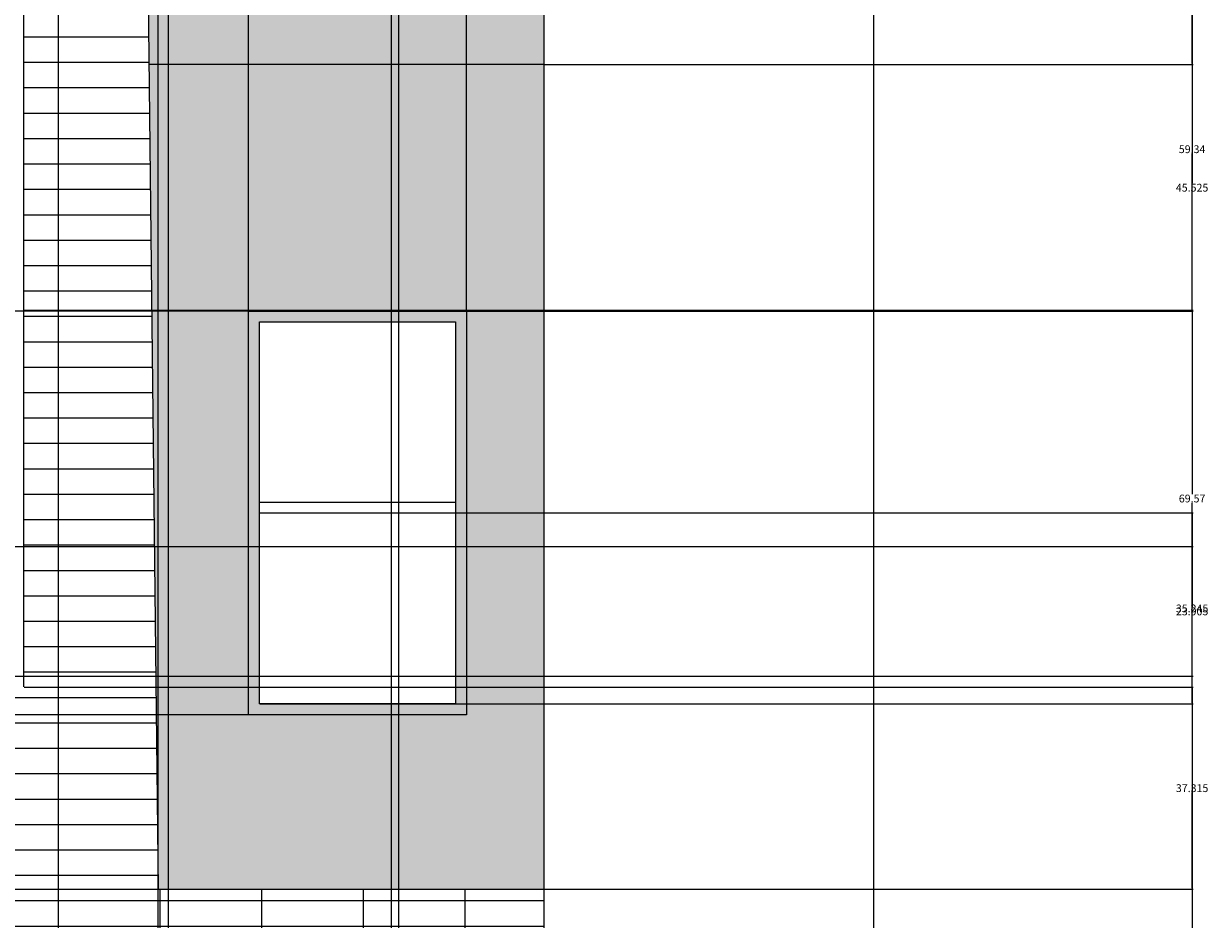
# Model space of a CAD drawing. Units: inches. Extents: x 241 to 943, y 109 to 1396.
# Tile 33 of 34: x 725 to 943, y 1065 to 1231. Entities that reach past the tile are written whole.
import ezdxf

# ---------------------------------------------------------------- set-up
doc = ezdxf.new("R2010")
doc.units = ezdxf.units.IN
doc.header["$MEASUREMENT"] = 0
for name, color, linetype, lineweight in [('A-ANNO-DIMS', 2, 'Continuous', 18), ('A-ELEV', 7, 'Continuous', 25), ('A-ELEV-SHAD', 9, 'Continuous', 13), ('A-GLAZ', 4, 'Continuous', 18), ('A-GLAZ-PATT', 18, 'Continuous', 13), ('A-WALL-PATT', 8, 'Continuous', 13)]:
    doc.layers.add(name, color=color, linetype=linetype, lineweight=lineweight)
doc.styles.get("Standard").update_dxf_attribs({"font": 'arial.ttf'})
doc.dimstyles.get("Standard").update_dxf_attribs({"dimtxt": 1.4375, "dimasz": 0.18, "dimexe": 0.18, "dimexo": 0.0625, "dimgap": 0.09, "dimtad": 0, "dimtih": 1, "dimtoh": 1, "dimdec": 4, "dimzin": 0, "dimdsep": 46, "dimlunit": 4, "dimtxsty": 'Standard', "dimcen": 0.09, "dimadec": 0, "dimazin": 0, "dimtfac": 1, "dimtdec": 4, "dimtofl": 0, "dimtmove": 0, "dimatfit": 3, "dimfxl": 1, "dimtolj": 1, "dimtzin": 0, "dimarcsym": 0})

# ---------------------------------------------------------------- blocks, each defined once
blk = doc.blocks.new('*D6')
at = {"layer": 'A-ANNO-DIMS', "color": 0, "lineweight": -2, "transparency": 16777216}
for p, q in [((820.84, 232.89), (820.84, 1395.05)), ((821.02, 1394.87), (848.73, 1394.87)), ((881.49, 1394.87), (853.77, 1394.87)), ((881.67, 232.89), (881.67, 1395.05))]:
    blk.add_line(p, q, dxfattribs=at)
at = {"layer": 'A-ANNO-DIMS', "color": 0, "transparency": 16777216}
for points in [[(821.02, 1394.9), (821.02, 1394.84), (820.84, 1394.87)], [(881.49, 1394.9), (881.49, 1394.84), (881.67, 1394.87)]]:
    blk.add_solid(points, dxfattribs=at)
at = {"layer": 'Defpoints', "color": 0, "transparency": 16777216}
for p in [(881.67, 1394.87), (820.84, 232.83), (881.67, 232.83)]:
    blk.add_point(p, dxfattribs=at)
at = {"layer": 'A-ANNO-DIMS', "color": 0, "transparency": 16777216, "insert": (851.25, 1394.87), "char_height": 1.438, "attachment_point": 5}
blk.add_mtext('\\A1;60.83', dxfattribs=at)
blk = doc.blocks.new('*D14')
at = {"layer": 'A-ANNO-DIMS', "color": 0, "lineweight": -2, "transparency": 16777216}
for p, q in [((667.39, 290.06), (667.39, 1395.05)), ((667.57, 1394.87), (727.7, 1394.87)), ((793.85, 1394.87), (733.72, 1394.87)), ((794.03, 290.06), (794.03, 1395.05))]:
    blk.add_line(p, q, dxfattribs=at)
at = {"layer": 'A-ANNO-DIMS', "color": 0, "transparency": 16777216}
for points in [[(667.57, 1394.9), (667.57, 1394.84), (667.39, 1394.87)], [(793.85, 1394.9), (793.85, 1394.84), (794.03, 1394.87)]]:
    blk.add_solid(points, dxfattribs=at)
at = {"layer": 'Defpoints', "color": 0, "transparency": 16777216}
for p in [(794.03, 1394.87), (667.39, 290), (794.03, 290)]:
    blk.add_point(p, dxfattribs=at)
at = {"layer": 'A-ANNO-DIMS', "color": 0, "transparency": 16777216, "insert": (730.71, 1394.87), "char_height": 1.438, "attachment_point": 5}
blk.add_mtext('\\A1;126.63', dxfattribs=at)
blk = doc.blocks.new('*D15')
at = {"layer": 'A-ANNO-DIMS', "color": 0, "lineweight": -2, "transparency": 16777216}
for p, q in [((794.03, 290.06), (794.03, 1395.05)), ((794.21, 1394.87), (805.04, 1394.87)), ((820.66, 1394.87), (809.82, 1394.87)), ((820.84, 232.89), (820.84, 1395.05))]:
    blk.add_line(p, q, dxfattribs=at)
at = {"layer": 'A-ANNO-DIMS', "color": 0, "transparency": 16777216}
for points in [[(794.21, 1394.9), (794.21, 1394.84), (794.03, 1394.87)], [(820.66, 1394.9), (820.66, 1394.84), (820.84, 1394.87)]]:
    blk.add_solid(points, dxfattribs=at)
at = {"layer": 'Defpoints', "color": 0, "transparency": 16777216}
for p in [(820.84, 1394.87), (794.03, 290), (820.84, 232.83)]:
    blk.add_point(p, dxfattribs=at)
at = {"layer": 'A-ANNO-DIMS', "color": 0, "transparency": 16777216, "insert": (807.43, 1394.87), "char_height": 1.438, "attachment_point": 5}
blk.add_mtext('\\A1;26.81', dxfattribs=at)
blk = doc.blocks.new('*D42')
at = {"layer": 'A-ANNO-DIMS', "color": 0, "lineweight": -2, "transparency": 16777216}
for p, q in [((820.9, 1275.91), (940.6, 1275.91)), ((940.42, 1275.73), (940.42, 1250.31)), ((940.42, 1223.24), (940.42, 1248.66)), ((820.9, 1223.06), (940.6, 1223.06))]:
    blk.add_line(p, q, dxfattribs=at)
at = {"layer": 'A-ANNO-DIMS', "color": 0, "transparency": 16777216}
for points in [[(940.39, 1275.73), (940.45, 1275.73), (940.42, 1275.91)], [(940.39, 1223.24), (940.45, 1223.24), (940.42, 1223.06)]]:
    blk.add_solid(points, dxfattribs=at)
at = {"layer": 'Defpoints', "color": 0, "transparency": 16777216}
for p in [(820.84, 1275.91), (940.42, 1275.91), (820.84, 1223.06)]:
    blk.add_point(p, dxfattribs=at)
at = {"layer": 'A-ANNO-DIMS', "color": 0, "transparency": 16777216, "insert": (940.42, 1249.49), "char_height": 1.438, "attachment_point": 5}
blk.add_mtext('\\A1;52.85', dxfattribs=at)
blk = doc.blocks.new('*D49')
at = {"layer": 'A-ANNO-DIMS', "color": 0, "lineweight": -2, "transparency": 16777216}
for p, q in [((766.24, 1177.54), (244.31, 1177.54)), ((244.49, 1177.36), (244.49, 1141.12)), ((244.49, 1103.23), (244.49, 1139.47)), ((766.24, 1103.05), (244.31, 1103.05))]:
    blk.add_line(p, q, dxfattribs=at)
at = {"layer": 'A-ANNO-DIMS', "color": 0, "transparency": 16777216}
for points in [[(244.46, 1177.36), (244.52, 1177.36), (244.49, 1177.54)], [(244.46, 1103.23), (244.52, 1103.23), (244.49, 1103.05)]]:
    blk.add_solid(points, dxfattribs=at)
at = {"layer": 'Defpoints', "color": 0, "transparency": 16777216}
for p in [(244.49, 1177.54), (766.3, 1177.54), (766.3, 1103.05)]:
    blk.add_point(p, dxfattribs=at)
at = {"layer": 'A-ANNO-DIMS', "color": 0, "transparency": 16777216, "insert": (244.49, 1140.29), "char_height": 1.438, "attachment_point": 5}
blk.add_mtext('\\A1;74.49', dxfattribs=at)
blk = doc.blocks.new('*D53')
at = {"layer": 'A-ANNO-DIMS', "color": 0, "lineweight": -2, "transparency": 16777216}
for p, q in [((724.88, 1177.73), (940.6, 1177.73)), ((940.42, 1177.55), (940.42, 1143.78)), ((940.42, 1108.35), (940.42, 1142.13)), ((724.88, 1108.17), (940.6, 1108.17))]:
    blk.add_line(p, q, dxfattribs=at)
at = {"layer": 'A-ANNO-DIMS', "color": 0, "transparency": 16777216}
for points in [[(940.39, 1177.55), (940.45, 1177.55), (940.42, 1177.73)], [(940.39, 1108.35), (940.45, 1108.35), (940.42, 1108.17)]]:
    blk.add_solid(points, dxfattribs=at)
at = {"layer": 'Defpoints', "color": 0, "transparency": 16777216}
for p in [(724.82, 1177.73), (940.42, 1177.73), (724.82, 1108.17)]:
    blk.add_point(p, dxfattribs=at)
at = {"layer": 'A-ANNO-DIMS', "color": 0, "transparency": 16777216, "insert": (940.42, 1142.95), "char_height": 1.438, "attachment_point": 5}
blk.add_mtext('\\A1;69.57', dxfattribs=at)
blk = doc.blocks.new('*D54')
at = {"layer": 'A-ANNO-DIMS', "color": 0, "lineweight": -2, "transparency": 16777216}
for p, q in [((724.88, 1237.07), (940.6, 1237.07)), ((940.42, 1236.89), (940.42, 1208.23)), ((940.42, 1177.91), (940.42, 1206.58)), ((724.88, 1177.73), (940.6, 1177.73))]:
    blk.add_line(p, q, dxfattribs=at)
at = {"layer": 'A-ANNO-DIMS', "color": 0, "transparency": 16777216}
for points in [[(940.39, 1236.89), (940.45, 1236.89), (940.42, 1237.07)], [(940.39, 1177.91), (940.45, 1177.91), (940.42, 1177.73)]]:
    blk.add_solid(points, dxfattribs=at)
at = {"layer": 'Defpoints', "color": 0, "transparency": 16777216}
for p in [(724.82, 1237.07), (940.42, 1237.07), (724.82, 1177.73)]:
    blk.add_point(p, dxfattribs=at)
at = {"layer": 'A-ANNO-DIMS', "color": 0, "transparency": 16777216, "insert": (940.42, 1207.4), "char_height": 1.438, "attachment_point": 5}
blk.add_mtext('\\A1;59.34', dxfattribs=at)
blk = doc.blocks.new('*D58')
at = {"layer": 'A-ANNO-DIMS', "color": 0, "lineweight": -2, "transparency": 16777216}
for p, q in [((766.3, 1177.6), (766.3, 1395.05)), ((766.48, 1394.87), (783.88, 1394.87)), ((806.35, 1394.87), (788.95, 1394.87)), ((806.53, 1177.6), (806.53, 1395.05))]:
    blk.add_line(p, q, dxfattribs=at)
at = {"layer": 'A-ANNO-DIMS', "color": 0, "transparency": 16777216}
for points in [[(766.48, 1394.9), (766.48, 1394.84), (766.3, 1394.87)], [(806.35, 1394.9), (806.35, 1394.84), (806.53, 1394.87)]]:
    blk.add_solid(points, dxfattribs=at)
at = {"layer": 'Defpoints', "color": 0, "transparency": 16777216}
for p in [(806.53, 1394.87), (766.3, 1177.54), (806.53, 1177.54)]:
    blk.add_point(p, dxfattribs=at)
at = {"layer": 'A-ANNO-DIMS', "color": 0, "transparency": 16777216, "insert": (786.42, 1394.87), "char_height": 1.438, "attachment_point": 5}
blk.add_mtext('\\A1;40.22', dxfattribs=at)
blk = doc.blocks.new('*D63')
at = {"layer": 'A-ANNO-DIMS', "color": 0, "lineweight": -2, "transparency": 16777216}
for p, q in [((651.6, 568.89), (651.6, 1395.05)), ((651.78, 1394.87), (719.84, 1394.87)), ((792.51, 1394.87), (724.45, 1394.87)), ((792.69, 568.89), (792.69, 1395.05))]:
    blk.add_line(p, q, dxfattribs=at)
at = {"layer": 'A-ANNO-DIMS', "color": 0, "transparency": 16777216}
for points in [[(651.78, 1394.9), (651.78, 1394.84), (651.6, 1394.87)], [(792.51, 1394.9), (792.51, 1394.84), (792.69, 1394.87)]]:
    blk.add_solid(points, dxfattribs=at)
at = {"layer": 'Defpoints', "color": 0, "transparency": 16777216}
for p in [(792.69, 1394.87), (651.6, 568.83), (792.69, 568.83)]:
    blk.add_point(p, dxfattribs=at)
at = {"layer": 'A-ANNO-DIMS', "color": 0, "transparency": 16777216, "insert": (722.14, 1394.87), "char_height": 1.438, "attachment_point": 5}
blk.add_mtext('\\A1;141.1', dxfattribs=at)
blk = doc.blocks.new('*D64')
at = {"layer": 'A-ANNO-DIMS', "color": 0, "lineweight": -2, "transparency": 16777216}
for p, q in [((792.69, 568.89), (792.69, 1395.05)), ((792.87, 1394.87), (803.68, 1394.87)), ((820.66, 1394.87), (809.85, 1394.87)), ((820.84, 568.89), (820.84, 1395.05))]:
    blk.add_line(p, q, dxfattribs=at)
at = {"layer": 'A-ANNO-DIMS', "color": 0, "transparency": 16777216}
for points in [[(792.87, 1394.9), (792.87, 1394.84), (792.69, 1394.87)], [(820.66, 1394.9), (820.66, 1394.84), (820.84, 1394.87)]]:
    blk.add_solid(points, dxfattribs=at)
at = {"layer": 'Defpoints', "color": 0, "transparency": 16777216}
for p in [(820.84, 1394.87), (792.69, 568.83), (820.84, 568.83)]:
    blk.add_point(p, dxfattribs=at)
at = {"layer": 'A-ANNO-DIMS', "color": 0, "transparency": 16777216, "insert": (806.76, 1394.87), "char_height": 1.438, "attachment_point": 5}
blk.add_mtext('\\A1;28.146', dxfattribs=at)
blk = doc.blocks.new('*D66')
at = {"layer": 'A-ANNO-DIMS', "color": 0, "lineweight": -2, "transparency": 16777216}
for p, q in [((617.76, 702.85), (617.76, 1395.05)), ((617.94, 1394.87), (680.69, 1394.87)), ((749.45, 1394.87), (686.7, 1394.87)), ((749.63, 702.85), (749.63, 1395.05))]:
    blk.add_line(p, q, dxfattribs=at)
at = {"layer": 'A-ANNO-DIMS', "color": 0, "transparency": 16777216}
for points in [[(617.94, 1394.9), (617.94, 1394.84), (617.76, 1394.87)], [(749.45, 1394.9), (749.45, 1394.84), (749.63, 1394.87)]]:
    blk.add_solid(points, dxfattribs=at)
at = {"layer": 'Defpoints', "color": 0, "transparency": 16777216}
for p in [(749.63, 1394.87), (617.76, 702.79), (749.63, 702.79)]:
    blk.add_point(p, dxfattribs=at)
at = {"layer": 'A-ANNO-DIMS', "color": 0, "transparency": 16777216, "insert": (683.7, 1394.87), "char_height": 1.438, "attachment_point": 5}
blk.add_mtext('\\A1;131.87', dxfattribs=at)
blk = doc.blocks.new('*D68')
at = {"layer": 'A-ANNO-DIMS', "color": 0, "lineweight": -2, "transparency": 16777216}
for p, q in [((617.76, 841.6), (617.76, 1395.05)), ((617.94, 1394.87), (702.22, 1394.87)), ((792.51, 1394.87), (708.23, 1394.87)), ((792.69, 841.6), (792.69, 1395.05))]:
    blk.add_line(p, q, dxfattribs=at)
at = {"layer": 'A-ANNO-DIMS', "color": 0, "transparency": 16777216}
for points in [[(617.94, 1394.9), (617.94, 1394.84), (617.76, 1394.87)], [(792.51, 1394.9), (792.51, 1394.84), (792.69, 1394.87)]]:
    blk.add_solid(points, dxfattribs=at)
at = {"layer": 'Defpoints', "color": 0, "transparency": 16777216}
for p in [(792.69, 1394.87), (617.76, 841.54), (792.69, 841.54)]:
    blk.add_point(p, dxfattribs=at)
at = {"layer": 'A-ANNO-DIMS', "color": 0, "transparency": 16777216, "insert": (705.23, 1394.87), "char_height": 1.438, "attachment_point": 5}
blk.add_mtext('\\A1;174.93', dxfattribs=at)
blk = doc.blocks.new('*D70')
at = {"layer": 'A-ANNO-DIMS', "color": 0, "lineweight": -2, "transparency": 16777216}
for p, q in [((603.87, 1009.6), (603.87, 1395.05)), ((604.05, 1394.87), (674.69, 1394.87)), ((751.33, 1394.87), (680.69, 1394.87)), ((751.51, 1009.6), (751.51, 1395.05))]:
    blk.add_line(p, q, dxfattribs=at)
at = {"layer": 'A-ANNO-DIMS', "color": 0, "transparency": 16777216}
for points in [[(604.05, 1394.9), (604.05, 1394.84), (603.87, 1394.87)], [(751.33, 1394.9), (751.33, 1394.84), (751.51, 1394.87)]]:
    blk.add_solid(points, dxfattribs=at)
at = {"layer": 'Defpoints', "color": 0, "transparency": 16777216}
for p in [(751.51, 1394.87), (603.87, 1009.54), (751.51, 1009.54)]:
    blk.add_point(p, dxfattribs=at)
at = {"layer": 'A-ANNO-DIMS', "color": 0, "transparency": 16777216, "insert": (677.69, 1394.87), "char_height": 1.438, "attachment_point": 5}
blk.add_mtext('\\A1;147.64', dxfattribs=at)
blk = doc.blocks.new('*D71')
at = {"layer": 'A-ANNO-DIMS', "color": 0, "lineweight": -2, "transparency": 16777216}
for p, q in [((751.51, 902.92), (751.51, 1395.05)), ((751.69, 1394.87), (783.65, 1394.87)), ((820.66, 1394.87), (788.69, 1394.87)), ((820.84, 902.92), (820.84, 1395.05))]:
    blk.add_line(p, q, dxfattribs=at)
at = {"layer": 'A-ANNO-DIMS', "color": 0, "transparency": 16777216}
for points in [[(751.69, 1394.9), (751.69, 1394.84), (751.51, 1394.87)], [(820.66, 1394.9), (820.66, 1394.84), (820.84, 1394.87)]]:
    blk.add_solid(points, dxfattribs=at)
at = {"layer": 'Defpoints', "color": 0, "transparency": 16777216}
for p in [(820.84, 1394.87), (751.51, 902.85), (820.84, 902.85)]:
    blk.add_point(p, dxfattribs=at)
at = {"layer": 'A-ANNO-DIMS', "color": 0, "transparency": 16777216, "insert": (786.17, 1394.87), "char_height": 1.438, "attachment_point": 5}
blk.add_mtext('\\A1;69.33', dxfattribs=at)
blk = doc.blocks.new('*D84')
at = {"layer": 'A-ANNO-DIMS', "color": 0, "lineweight": -2, "transparency": 16777216}
for p, q in [((749.63, 702.85), (749.63, 1395.05)), ((749.81, 1394.87), (782.73, 1394.87)), ((820.66, 1394.87), (787.74, 1394.87)), ((820.84, 736.89), (820.84, 1395.05))]:
    blk.add_line(p, q, dxfattribs=at)
at = {"layer": 'A-ANNO-DIMS', "color": 0, "transparency": 16777216}
for points in [[(749.81, 1394.9), (749.81, 1394.84), (749.63, 1394.87)], [(820.66, 1394.9), (820.66, 1394.84), (820.84, 1394.87)]]:
    blk.add_solid(points, dxfattribs=at)
at = {"layer": 'Defpoints', "color": 0, "transparency": 16777216}
for p in [(820.84, 1394.87), (820.84, 736.83), (749.63, 702.79)]:
    blk.add_point(p, dxfattribs=at)
at = {"layer": 'A-ANNO-DIMS', "color": 0, "transparency": 16777216, "insert": (785.24, 1394.87), "char_height": 1.438, "attachment_point": 5}
blk.add_mtext('\\A1;71.20', dxfattribs=at)
blk = doc.blocks.new('*D88')
at = {"layer": 'A-ANNO-DIMS', "color": 0, "lineweight": -2, "transparency": 16777216}
for p, q in [((724.88, 1108.17), (940.6, 1108.17)), ((940.42, 1107.99), (940.42, 1059.68)), ((940.42, 1009.72), (940.42, 1058.03)), ((751.57, 1009.54), (940.6, 1009.54))]:
    blk.add_line(p, q, dxfattribs=at)
at = {"layer": 'A-ANNO-DIMS', "color": 0, "transparency": 16777216}
for points in [[(940.39, 1107.99), (940.45, 1107.99), (940.42, 1108.17)], [(940.39, 1009.72), (940.45, 1009.72), (940.42, 1009.54)]]:
    blk.add_solid(points, dxfattribs=at)
at = {"layer": 'Defpoints', "color": 0, "transparency": 16777216}
for p in [(724.82, 1108.17), (940.42, 1108.17), (751.51, 1009.54)]:
    blk.add_point(p, dxfattribs=at)
at = {"layer": 'A-ANNO-DIMS', "color": 0, "transparency": 16777216, "insert": (940.42, 1058.85), "char_height": 1.438, "attachment_point": 5}
blk.add_mtext('\\A1;98.63', dxfattribs=at)
blk = doc.blocks.new('*D94')
at = {"layer": 'A-ANNO-DIMS', "color": 0, "lineweight": -2, "transparency": 16777216}
for p, q in [((747.76, 1275.98), (747.76, 1395.05)), ((747.94, 1394.87), (754.03, 1394.87)), ((766.12, 1394.87), (760.04, 1394.87)), ((766.3, 1103.11), (766.3, 1395.05))]:
    blk.add_line(p, q, dxfattribs=at)
at = {"layer": 'A-ANNO-DIMS', "color": 0, "transparency": 16777216}
for points in [[(747.94, 1394.9), (747.94, 1394.84), (747.76, 1394.87)], [(766.12, 1394.9), (766.12, 1394.84), (766.3, 1394.87)]]:
    blk.add_solid(points, dxfattribs=at)
at = {"layer": 'Defpoints', "color": 0, "transparency": 16777216}
for p in [(766.3, 1394.87), (747.76, 1275.91), (766.3, 1103.05)]:
    blk.add_point(p, dxfattribs=at)
at = {"layer": 'A-ANNO-DIMS', "color": 0, "transparency": 16777216, "insert": (757.03, 1394.87), "char_height": 1.438, "attachment_point": 5}
blk.add_mtext('\\A1;18.546', dxfattribs=at)
blk = doc.blocks.new('*D95')
at = {"layer": 'A-ANNO-DIMS', "color": 0, "lineweight": -2, "transparency": 16777216}
for p, q in [((724.88, 1108.17), (940.6, 1108.17)), ((940.42, 1107.99), (940.42, 1090.34)), ((940.42, 1071.03), (940.42, 1088.69)), ((508.37, 1070.85), (940.6, 1070.85))]:
    blk.add_line(p, q, dxfattribs=at)
at = {"layer": 'A-ANNO-DIMS', "color": 0, "transparency": 16777216}
for points in [[(940.39, 1107.99), (940.45, 1107.99), (940.42, 1108.17)], [(940.39, 1071.03), (940.45, 1071.03), (940.42, 1070.85)]]:
    blk.add_solid(points, dxfattribs=at)
at = {"layer": 'Defpoints', "color": 0, "transparency": 16777216}
for p in [(724.82, 1108.17), (940.42, 1108.17), (508.31, 1070.85)]:
    blk.add_point(p, dxfattribs=at)
at = {"layer": 'A-ANNO-DIMS', "color": 0, "transparency": 16777216, "insert": (940.42, 1089.51), "char_height": 1.438, "attachment_point": 5}
blk.add_mtext('\\A1;37.315', dxfattribs=at)
blk = doc.blocks.new('*D96')
at = {"layer": 'A-ANNO-DIMS', "color": 0, "lineweight": -2, "transparency": 16777216}
for p, q in [((820.9, 1223.06), (940.6, 1223.06)), ((940.42, 1222.88), (940.42, 1201.12)), ((940.42, 1177.72), (940.42, 1199.48)), ((806.59, 1177.54), (940.6, 1177.54))]:
    blk.add_line(p, q, dxfattribs=at)
at = {"layer": 'A-ANNO-DIMS', "color": 0, "transparency": 16777216}
for points in [[(940.39, 1222.88), (940.45, 1222.88), (940.42, 1223.06)], [(940.39, 1177.72), (940.45, 1177.72), (940.42, 1177.54)]]:
    blk.add_solid(points, dxfattribs=at)
at = {"layer": 'Defpoints', "color": 0, "transparency": 16777216}
for p in [(820.84, 1223.06), (940.42, 1223.06), (806.53, 1177.54)]:
    blk.add_point(p, dxfattribs=at)
at = {"layer": 'A-ANNO-DIMS', "color": 0, "transparency": 16777216, "insert": (940.42, 1200.3), "char_height": 1.438, "attachment_point": 5}
blk.add_mtext('\\A1;45.525', dxfattribs=at)
blk = doc.blocks.new('*D109')
at = {"layer": 'A-ANNO-DIMS', "color": 0, "lineweight": -2, "transparency": 16777216}
for p, q in [((682.87, 1110.23), (682.87, 1395.05)), ((683.05, 1394.87), (701.31, 1394.87)), ((724.64, 1394.87), (706.39, 1394.87)), ((724.82, 1108.23), (724.82, 1395.05))]:
    blk.add_line(p, q, dxfattribs=at)
at = {"layer": 'A-ANNO-DIMS', "color": 0, "transparency": 16777216}
for points in [[(683.05, 1394.9), (683.05, 1394.84), (682.87, 1394.87)], [(724.64, 1394.9), (724.64, 1394.84), (724.82, 1394.87)]]:
    blk.add_solid(points, dxfattribs=at)
at = {"layer": 'Defpoints', "color": 0, "transparency": 16777216}
for p in [(724.82, 1394.87), (682.87, 1110.17), (724.82, 1108.17)]:
    blk.add_point(p, dxfattribs=at)
at = {"layer": 'A-ANNO-DIMS', "color": 0, "transparency": 16777216, "insert": (703.85, 1394.87), "char_height": 1.438, "attachment_point": 5}
blk.add_mtext('\\A1;41.94', dxfattribs=at)
blk = doc.blocks.new('*D111')
at = {"layer": 'A-ANNO-DIMS', "color": 0, "lineweight": -2, "transparency": 16777216}
for p, q in [((622.58, 1134.07), (940.6, 1134.07)), ((940.42, 1133.89), (940.42, 1122.95)), ((940.42, 1110.35), (940.42, 1121.3)), ((622.58, 1110.17), (940.6, 1110.17))]:
    blk.add_line(p, q, dxfattribs=at)
at = {"layer": 'A-ANNO-DIMS', "color": 0, "transparency": 16777216}
for points in [[(940.39, 1133.89), (940.45, 1133.89), (940.42, 1134.07)], [(940.39, 1110.35), (940.45, 1110.35), (940.42, 1110.17)]]:
    blk.add_solid(points, dxfattribs=at)
at = {"layer": 'Defpoints', "color": 0, "transparency": 16777216}
for p in [(622.52, 1134.07), (940.42, 1134.07), (622.52, 1110.17)]:
    blk.add_point(p, dxfattribs=at)
at = {"layer": 'A-ANNO-DIMS', "color": 0, "transparency": 16777216, "insert": (940.42, 1122.12), "char_height": 1.438, "attachment_point": 5}
blk.add_mtext('\\A1;23.905', dxfattribs=at)
blk = doc.blocks.new('*D112')
at = {"layer": 'A-ANNO-DIMS', "color": 0, "lineweight": -2, "transparency": 16777216}
for p, q in [((768.37, 1140.29), (940.6, 1140.29)), ((940.42, 1140.11), (940.42, 1123.49)), ((940.42, 1105.23), (940.42, 1121.85)), ((768.37, 1105.05), (940.6, 1105.05))]:
    blk.add_line(p, q, dxfattribs=at)
at = {"layer": 'A-ANNO-DIMS', "color": 0, "transparency": 16777216}
for points in [[(940.39, 1140.11), (940.45, 1140.11), (940.42, 1140.29)], [(940.39, 1105.23), (940.45, 1105.23), (940.42, 1105.05)]]:
    blk.add_solid(points, dxfattribs=at)
at = {"layer": 'Defpoints', "color": 0, "transparency": 16777216}
for p in [(768.3, 1140.29), (940.42, 1140.29), (768.3, 1105.05)]:
    blk.add_point(p, dxfattribs=at)
at = {"layer": 'A-ANNO-DIMS', "color": 0, "transparency": 16777216, "insert": (940.42, 1122.67), "char_height": 1.438, "attachment_point": 5}
blk.add_mtext('\\A1;35.245', dxfattribs=at)
blk = doc.blocks.new('*D117')
at = {"layer": 'A-ANNO-DIMS', "color": 0, "lineweight": -2, "transparency": 16777216}
for p, q in [((712.58, 902.92), (712.58, 1395.05)), ((712.76, 1394.87), (729.54, 1394.87)), ((751.33, 1394.87), (734.55, 1394.87)), ((751.51, 902.92), (751.51, 1395.05))]:
    blk.add_line(p, q, dxfattribs=at)
at = {"layer": 'A-ANNO-DIMS', "color": 0, "transparency": 16777216}
for points in [[(712.76, 1394.9), (712.76, 1394.84), (712.58, 1394.87)], [(751.33, 1394.9), (751.33, 1394.84), (751.51, 1394.87)]]:
    blk.add_solid(points, dxfattribs=at)
at = {"layer": 'Defpoints', "color": 0, "transparency": 16777216}
for p in [(751.51, 1394.87), (712.58, 902.85), (751.51, 902.85)]:
    blk.add_point(p, dxfattribs=at)
at = {"layer": 'A-ANNO-DIMS', "color": 0, "transparency": 16777216, "insert": (732.05, 1394.87), "char_height": 1.438, "attachment_point": 5}
blk.add_mtext('\\A1;38.92', dxfattribs=at)

msp = doc.modelspace()

# ---------------------------------------------------------------- hatches: boundary and pattern name
at = {"layer": 'A-ELEV-SHAD'}
h = msp.add_hatch(color=256, dxfattribs=at)
h.dxf.hatch_style = 1
h.paths.add_polyline_path([(508.3064, 1070.8538), (377.0391, 1070.8538), (377.0391, 1009.5382), (508.3064, 1009.5382)])
h.paths.add_polyline_path([(508.3064, 1238.8538), (377.0391, 1238.8538), (377.0391, 1177.5382), (508.3064, 1177.5382)])
h.paths.add_polyline_path([(581.3632, 902.8538), (568.1348, 902.8538), (553.5166, 902.8538), (377.0391, 902.8538), (377.0391, 841.5382), (553.5166, 841.5382), (564.8076, 841.5382), (581.3632, 841.5382)])
h.paths.add_polyline_path([(820.8374, 1275.9142), (747.7579, 1275.9142), (747.7579, 1238.8538), (820.8374, 1238.8538)])
h.paths.add_polyline_path([(820.8374, 1238.8538), (747.7579, 1238.8538), (747.9341, 1223.0633), (820.8374, 1223.0633)])
h.paths.add_polyline_path([(396.3125, 841.5382), (377.0391, 841.5382), (377.0391, 734.8538), (389.0429, 734.8538), (389.0429, 735.188), (389.0429, 773.4916), (396.3125, 773.4916), (396.3125, 780.5808), (390.5597, 780.5808), (388.0428, 780.5808, -1), (388.0428, 782.5808), (390.5597, 782.5808), (396.3125, 782.5808)])
h = msp.add_hatch(color=256, dxfattribs=at)
h.dxf.hatch_style = 1
h.paths.add_polyline_path([(820.8374, 1223.0633), (747.9341, 1223.0633), (749.6328, 1070.8538), (820.8374, 1070.8538)])
h.paths.add_polyline_path([(806.5268, 1177.5382), (806.5268, 1103.0477), (766.3038, 1103.0477), (766.3038, 1177.5382)], flags=16)
h.paths.add_polyline_path([(804.5268, 1175.5382), (804.5268, 1105.0477), (768.3038, 1105.0477), (768.3038, 1175.5382)], flags=0)
h = msp.add_hatch(color=256, dxfattribs=at)
h.dxf.hatch_style = 1
h.paths.add_polyline_path([(804.5268, 1142.2929), (768.3038, 1142.2929), (768.3038, 1140.2929), (804.5268, 1140.2929)], flags=0)
h.paths.add_polyline_path([(806.5268, 1177.5382), (766.3038, 1177.5382), (766.3038, 1103.0477), (806.5268, 1103.0477)])
h.paths.add_polyline_path([(768.3038, 1175.5382), (804.5268, 1175.5382), (804.5268, 1105.0477), (768.3038, 1105.0477)], flags=16)
h.paths.add_polyline_path([(643.4534, 1136.0739), (622.521, 1136.0739), (622.521, 1134.0739), (643.4534, 1134.0739)])
h.paths.add_polyline_path([(622.521, 1175.7336), (620.521, 1175.7336), (620.521, 1110.1686), (622.521, 1110.1686)])
h.paths.add_polyline_path([(565.947, 1151.5772), (535.952, 1151.5772), (535.952, 1149.5772), (565.947, 1149.5772)])
at = {"layer": 'A-GLAZ-PATT'}
h = msp.add_hatch(dxfattribs=at)
h.set_pattern_fill('ANSI31', color=256, scale=34, angle=45)
h.paths.add_polyline_path([(486.3418, 786.9154), (413.1187, 786.9154), (413.1187, 761.2284), (486.3418, 761.2284)])
h.paths.add_polyline_path([(486.3418, 954.9154), (413.1187, 954.9154), (413.1187, 929.2284), (486.3418, 929.2284)])
h.paths.add_polyline_path([(462.1074, 289.6933), (390.895, 289.6933), (390.895, 277.4626), (390.895, 274.3507), (462.1074, 274.3507), (462.1074, 277.4626)])
h.paths.add_polyline_path([(500.3323, 289.6933), (479.596, 289.6933), (479.596, 274.3507), (500.3323, 274.3507)])
h.paths.add_polyline_path([(450.9259, 566.8295), (426.1086, 566.8295), (426.1086, 498.4395), (446.4348, 498.4395), (446.4348, 519.3754), (450.9259, 519.3754), (450.9259, 525.3816), (445.5808, 525.3816, -1), (445.5808, 527.3816), (450.9259, 527.3816)])
h.paths.add_polyline_path([(563.2023, 508.9074), (534.1778, 508.9074), (508.1906, 508.9074), (508.1906, 498.4395), (563.2023, 498.4395)])
h.paths.add_polyline_path([(747.6328, 700.7912), (712.0171, 700.7912), (712.0171, 628.4013), (747.6328, 628.4013)])
h.paths.add_polyline_path([(446.4348, 643.7483), (426.1086, 643.7483), (426.1086, 630.4013), (446.4348, 630.4013)])
h.paths.add_polyline_path([(564.8076, 841.5382), (553.5166, 841.5382), (508.3064, 841.5382), (508.3064, 782.5808), (564.8076, 782.5808)])
h.paths.add_polyline_path([(564.8076, 780.5808), (508.3064, 780.5808), (508.3064, 773.4916), (564.8076, 773.4916)])
h.paths.add_polyline_path([(792.691, 762.5799), (759.6248, 762.5799), (759.6248, 736.9235), (759.6248, 734.8538), (792.691, 734.8538)])
h.paths.add_polyline_path([(564.8076, 1009.5382), (553.5166, 1009.5382), (508.3064, 1009.5382), (508.3064, 950.5808), (562.3033, 950.5808, -1), (562.3033, 948.5808), (508.3064, 948.5808), (508.3064, 941.4916), (564.8076, 941.4916)])
h.paths.add_polyline_path([(486.3418, 1122.9154), (413.1187, 1122.9154), (413.1187, 1097.2284), (486.3418, 1097.2284)])
at = {"layer": 'A-WALL-PATT'}
h = msp.add_hatch(dxfattribs=at)
h.set_pattern_fill('GRATE', color=256, scale=150)
h.paths.add_polyline_path([(747.7579, 1238.8538), (747.7579, 1275.9142), (747.7579, 1336.1154), (508.3064, 1336.1154), (508.3064, 1275.9142), (508.3064, 1238.8538), (508.3064, 1177.5382), (508.3064, 1109.4916), (508.3064, 1070.8538), (553.5166, 1070.8538), (749.6328, 1070.8538)])
h.paths.add_polyline_path([(533.952, 1108.1686), (533.952, 1177.7336), (533.952, 1303.0286), (724.819, 1303.0286), (724.819, 1108.1686)], flags=16)
h.paths.add_polyline_path([(535.952, 1110.1686), (535.952, 1175.7336), (722.819, 1175.7336), (722.819, 1110.1686)], flags=0)
h.paths.add_polyline_path([(643.4534, 1134.0739), (622.521, 1134.0739), (622.521, 1136.0739), (643.4534, 1136.0739)], flags=0)
h.paths.add_polyline_path([(617.7594, 568.8295), (617.7594, 734.8538), (377.0391, 734.8538), (377.0391, 566.8538), (377.0391, 400.8295), (417.0913, 400.8295), (618.9643, 400.8295)])
h.paths.add_polyline_path([(424.1086, 496.4395), (424.1086, 568.8295), (565.2023, 568.8295), (565.2023, 496.4395)], flags=16)
h.paths.add_polyline_path([(426.1086, 498.4395), (426.1086, 566.8295), (563.2023, 566.8295), (563.2023, 508.9074), (563.2023, 498.4395)], flags=0)
h.paths.add_polyline_path([(508.0803, 508.9074), (508.0803, 519.3754), (450.9259, 519.3754), (450.9259, 525.3816), (445.5808, 525.3816, -1), (445.5808, 527.3816), (450.9259, 527.3816), (450.9259, 566.8295), (508.0803, 566.8295), (537.4269, 566.8295), (537.4269, 508.9074)], flags=0)
h.paths.add_polyline_path([(506.0803, 521.3754), (452.9259, 521.3754), (452.9259, 564.8295), (506.0803, 564.8295)], flags=0)
h.paths.add_polyline_path([(424.1086, 628.4013), (424.1086, 700.7912), (592.9542, 700.7912), (592.9542, 628.4013)], flags=16)
h.paths.add_polyline_path([(426.1086, 630.4013), (426.1086, 698.7912), (590.8792, 698.7912), (590.8792, 630.4013)], flags=0)
h.paths.add_polyline_path([(508.1906, 651.3371), (508.0803, 651.3371), (450.9259, 651.3371), (428.0291, 651.3371), (428.0291, 698.7912), (451.9767, 698.7912), (508.0803, 698.7912), (537.4269, 698.7912), (563.2023, 698.7912), (563.2023, 659.3434), (563.9297, 659.3434), (563.9297, 651.3371)], flags=0)
h.paths.add_polyline_path([(506.0803, 653.3371), (452.9259, 653.3371), (452.9259, 657.3434), (445.5808, 657.3434, -1), (445.5808, 659.3434), (452.9259, 659.3434), (452.9259, 696.7912), (506.0803, 696.7912)], flags=0)
h = msp.add_hatch(dxfattribs=at)
h.set_pattern_fill('GRATE', color=256, scale=150)
h.paths.add_polyline_path([(820.8374, 1070.8538), (749.6328, 1070.8538), (553.5166, 1070.8538), (508.3064, 1070.8538), (508.3064, 1009.5382), (553.5166, 1009.5382), (564.8076, 1009.5382), (603.8694, 1009.5382), (751.5078, 1009.5382), (751.5078, 902.8538), (603.8694, 902.8538), (603.8694, 1009.5382), (564.8076, 1009.5382), (564.8076, 941.4916), (568.1348, 941.4916), (568.1348, 902.8538), (581.3632, 902.8538), (581.3632, 841.5382), (564.8076, 841.5382), (564.8076, 782.5808), (605.9087, 782.5808, -1), (605.9087, 780.5808), (564.8076, 780.5808), (564.8076, 773.4916), (597.514, 773.4916), (607.8162, 773.4916), (607.8162, 734.8538), (617.7594, 734.8538), (617.7594, 841.5382), (792.691, 841.5382), (792.691, 734.8538), (617.7594, 734.8538), (617.7594, 702.7912), (749.6328, 702.7912), (749.6328, 626.4013), (617.7594, 626.4013), (617.7594, 568.8295), (820.8374, 568.8295), (820.8374, 736.8295), (820.8374, 902.8538)])

# ---------------------------------------------------------------- linework, layer by layer
at = {"layer": 'A-ELEV'}
for p, q in [((747.7579, 1238.8538), (749.6328, 1070.8538)), ((820.8374, 1070.8538), (820.8374, 1238.8538)), ((747.9341, 1223.0633), (820.8374, 1223.0633)), ((553.5166, 1070.8538), (749.6328, 1070.8538)), ((749.6328, 1070.8538), (820.8374, 1070.8538)), ((820.8374, 902.8538), (820.8374, 1070.8538))]:
    msp.add_line(p, q, dxfattribs=at)
at = {"layer": 'A-GLAZ'}
for p, q in [((768.3038, 1142.2929), (804.5268, 1142.2929)), ((768.3038, 1140.2929), (804.5268, 1140.2929))]:
    msp.add_line(p, q, dxfattribs=at)
for points in [[(766.3038, 1177.5382), (806.5268, 1177.5382), (806.5268, 1103.0477), (766.3038, 1103.0477)], [(768.3038, 1175.5382), (804.5268, 1175.5382), (804.5268, 1105.0477), (768.3038, 1105.0477)]]:
    msp.add_lwpolyline(points, close=True, dxfattribs=at)

# ---------------------------------------------------------------- dimensions: what is measured, and where the dimension line sits
at = {"layer": 'A-ANNO-DIMS'}
for base, p1, p2, override, picture, middle in [((751.5078, 1394.8654), (603.8694, 1009.5382), (751.5078, 1009.5382), {"dimdec": 2, "dimlfac": 1, "dimrnd": 0, "dimzin": 0, "dimdsep": 46, "dimlunit": 2}, '*D70', (677.6886, 1394.8654)), ((749.6328, 1394.8654), (617.7594, 702.7912), (749.6328, 702.7912), {"dimdec": 2, "dimlfac": 1, "dimrnd": 0, "dimzin": 0, "dimdsep": 46, "dimlunit": 2}, '*D66', (683.6961, 1394.8654)), ((792.691, 1394.8654), (617.7594, 841.5382), (792.691, 841.5382), {"dimdec": 2, "dimlfac": 1, "dimrnd": 0, "dimzin": 0, "dimdsep": 46, "dimlunit": 2}, '*D68', (705.2252, 1394.8654)), ((792.691, 1394.8654), (651.5974, 568.8295), (792.691, 568.8295), {"dimdec": 1, "dimlfac": 1, "dimrnd": 0, "dimzin": 0, "dimdsep": 46, "dimlunit": 2}, '*D63', (722.1442, 1394.8654)), ((794.0275, 1394.8654), (667.3935, 289.9984), (794.0275, 289.9984), {"dimdec": 2, "dimlfac": 1, "dimrnd": 0, "dimzin": 0, "dimdsep": 46, "dimlunit": 2}, '*D14', (730.7105, 1394.8654)), ((724.819, 1394.8654), (682.8748, 1110.1686), (724.819, 1108.1686), {"dimdec": 2, "dimlfac": 1, "dimrnd": 0, "dimzin": 0, "dimdsep": 46, "dimlunit": 2}, '*D109', (703.8469, 1394.8654)), ((751.5078, 1394.8654), (712.5839, 902.8538), (751.5078, 902.8538), {"dimdec": 2, "dimlfac": 1, "dimrnd": 0, "dimzin": 0, "dimdsep": 46, "dimlunit": 2}, '*D117', (732.0459, 1394.8654)), ((766.3038, 1394.8654), (747.7579, 1275.9142), (766.3038, 1103.0477), {"dimdec": 3, "dimlfac": 1, "dimrnd": 0, "dimzin": 0, "dimdsep": 46, "dimlunit": 2}, '*D94', (757.0309, 1394.8654)), ((820.8374, 1394.8654), (749.6328, 702.7912), (820.8374, 736.8295), {"dimdec": 2, "dimlfac": 1, "dimrnd": 0, "dimzin": 0, "dimdsep": 46, "dimlunit": 2}, '*D84', (785.2351, 1394.8654)), ((820.8374, 1394.8654), (751.5078, 902.8538), (820.8374, 902.8538), {"dimdec": 2, "dimlfac": 1, "dimrnd": 0, "dimzin": 0, "dimdsep": 46, "dimlunit": 2}, '*D71', (786.1726, 1394.8654)), ((806.5268, 1394.8654), (766.3038, 1177.5382), (806.5268, 1177.5382), {"dimdec": 2, "dimlfac": 1, "dimrnd": 0, "dimzin": 0, "dimdsep": 46, "dimlunit": 2}, '*D58', (786.4153, 1394.8654)), ((820.8374, 1394.8654), (792.691, 568.8295), (820.8374, 568.8295), {"dimdec": 3, "dimlfac": 1, "dimrnd": 0, "dimzin": 0, "dimdsep": 46, "dimlunit": 2}, '*D64', (806.7642, 1394.8654)), ((820.8374, 1394.8654), (794.0275, 289.9984), (820.8374, 232.8295), {"dimdec": 2, "dimlfac": 1, "dimrnd": 0, "dimzin": 0, "dimdsep": 46, "dimlunit": 2}, '*D15', (807.4324, 1394.8654)), ((881.667, 1394.8654), (820.8374, 232.8295), (881.667, 232.8295), {"dimdec": 2, "dimlfac": 1, "dimrnd": 0, "dimzin": 0, "dimdsep": 46, "dimlunit": 2}, '*D6', (851.2522, 1394.8654))]:
    dim = msp.add_linear_dim(base=base, p1=p1, p2=p2, dimstyle='Standard', override=override, dxfattribs=at)
    dim.commit()
    dim.dimension.update_dxf_attribs({"geometry": picture, "text_midpoint": middle})
for base, p1, p2, override, picture, middle in [((940.417, 1275.9142), (820.8374, 1223.0633), (820.8374, 1275.9142), {"dimdec": 2, "dimlfac": 1, "dimrnd": 0, "dimzin": 0, "dimdsep": 46, "dimlunit": 2}, '*D42', (940.417, 1249.4888)), ((940.417, 1237.0695), (724.819, 1177.7336), (724.819, 1237.0695), {"dimdec": 2, "dimlfac": 1, "dimrnd": 0, "dimzin": 0, "dimdsep": 46, "dimlunit": 2}, '*D54', (940.417, 1207.4016)), ((940.417, 1223.0633), (806.5268, 1177.5382), (820.8374, 1223.0633), {"dimdec": 3, "dimlfac": 1, "dimrnd": 0, "dimzin": 0, "dimdsep": 46, "dimlunit": 2}, '*D96', (940.417, 1200.3007)), ((244.4858, 1177.5382), (766.3038, 1103.0477), (766.3038, 1177.5382), {"dimdec": 2, "dimlfac": 1, "dimrnd": 0, "dimzin": 0, "dimdsep": 46, "dimlunit": 2}, '*D49', (244.4858, 1140.2929)), ((940.417, 1177.73365), (724.81903, 1108.16855), (724.81903, 1177.73365), {"dimdec": 2, "dimlfac": 1, "dimrnd": 0, "dimzin": 0, "dimdsep": 46, "dimlunit": 2}, '*D53', (940.417, 1142.9511)), ((940.417, 1140.2929), (768.3038, 1105.0477), (768.3038, 1140.2929), {"dimdec": 3, "dimlfac": 1, "dimrnd": 0, "dimzin": 0, "dimdsep": 46, "dimlunit": 2}, '*D112', (940.417, 1122.6703)), ((940.417, 1134.0739), (622.521, 1110.1686), (622.521, 1134.0739), {"dimdec": 3, "dimlfac": 1, "dimrnd": 0, "dimzin": 0, "dimdsep": 46, "dimlunit": 2}, '*D111', (940.417, 1122.1212)), ((940.417, 1108.1686), (508.3064, 1070.8538), (724.819, 1108.1686), {"dimdec": 3, "dimlfac": 1, "dimrnd": 0, "dimzin": 0, "dimdsep": 46, "dimlunit": 2}, '*D95', (940.417, 1089.5112)), ((940.417, 1108.1686), (751.5078, 1009.5382), (724.819, 1108.1686), {"dimdec": 2, "dimlfac": 1, "dimrnd": 0, "dimzin": 0, "dimdsep": 46, "dimlunit": 2}, '*D88', (940.417, 1058.8534))]:
    dim = msp.add_linear_dim(base=base, p1=p1, p2=p2, angle=90, dimstyle='Standard', override=override, dxfattribs=at)
    dim.commit()
    dim.dimension.update_dxf_attribs({"geometry": picture, "text_midpoint": middle})

doc.saveas('drawing.dxf')
